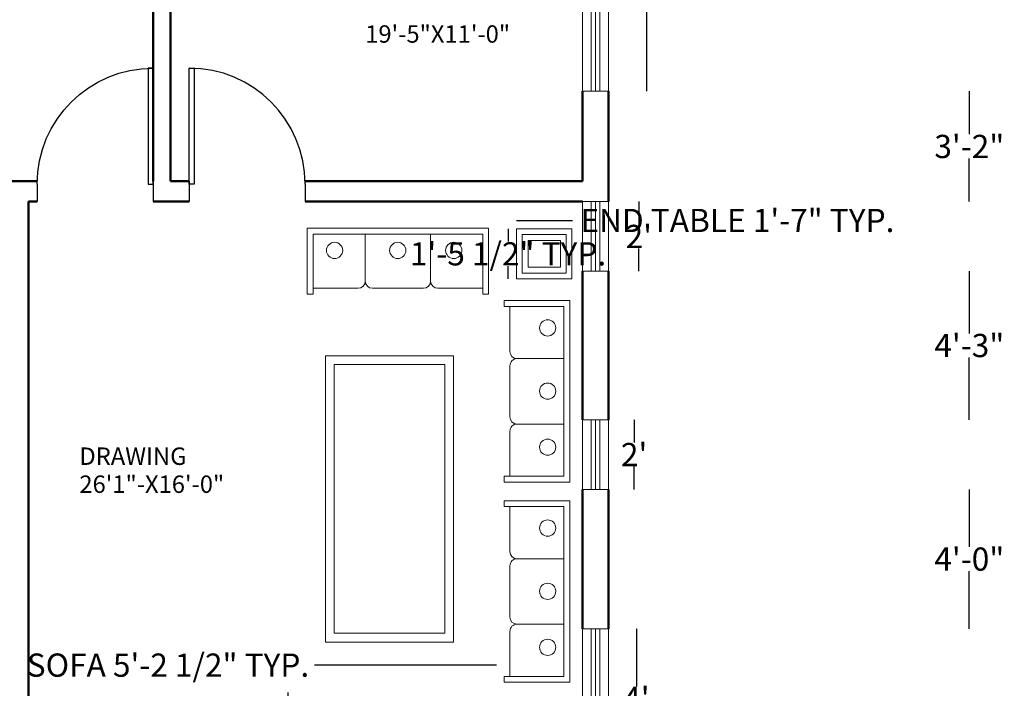
# Model space of a CAD drawing. Units: inches. Extents: x -135167 to -134597, y 156853 to 157819.
# Tile 4 of 5: x -134948 to -134608, y 157306 to 157537. Entities that reach past the tile are written whole.
import ezdxf

# ---------------------------------------------------------------- set-up
doc = ezdxf.new("R2010")
doc.units = ezdxf.units.IN
doc.header["$MEASUREMENT"] = 0
for name, color, linetype, lineweight in [('A-ANNO-DIMS', 4, 'Continuous', 18), ('A-AREA-IDEN', 76, 'Continuous', 25), ('A-FURN', 1, 'Continuous', 18), ('doors', 5, 'Continuous', 25), ('walls', 2, 'Continuous', 50), ('window', 6, 'Continuous', 18)]:
    doc.layers.add(name, color=color, linetype=linetype, lineweight=lineweight)
doc.styles.get("Standard").update_dxf_attribs({"font": 'arial.ttf'})
doc.dimstyles.get("Standard").update_dxf_attribs({"dimtxt": 8, "dimasz": 0.18, "dimexe": 0.18, "dimexo": 0.0625, "dimgap": 0.09, "dimtad": 0, "dimtih": 1, "dimtoh": 1, "dimdec": 0, "dimzin": 0, "dimdsep": 46, "dimlunit": 3, "dimtxsty": 'Standard', "dimblk": 'ARCHTICK', "dimcen": 0.09, "dimse1": 1, "dimse2": 1, "dimadec": 0, "dimazin": 0, "dimtfac": 1, "dimtdec": 0, "dimtofl": 0, "dimtmove": 0, "dimatfit": 3, "dimldrblk": 'DOTSMALL', "dimfxl": 1, "dimtolj": 1, "dimtzin": 0, "dimarcsym": 0})

# ---------------------------------------------------------------- blocks, each defined once
blk = doc.blocks.new('*U6')
for p, q in [((0, 0), (0, -6)), ((40, 0), (40, -6))]:
    blk.add_line(p, q)
blk.add_lwpolyline([(0, 0), (0, 40), (1.75, 40), (1.75, 0)], close=True)
blk.add_arc((0, 0), 40, 0, 90)
blk = doc.blocks.new('_ArchTick')
at = {"color": 0, "linetype": 'ByBlock', "const_width": 0.15}
blk.add_lwpolyline([(-0.5, -0.5), (0.5, 0.5)], dxfattribs=at)
blk = doc.blocks.new('*D25')
at = {"layer": 'A-ANNO-DIMS', "color": 0, "lineweight": -2, "transparency": 16777216}
for p, q in [((-134735.32, 157326.8), (-134735.32, 157306.89)), ((-134735.32, 157278.8), (-134735.32, 157298.71))]:
    blk.add_line(p, q, dxfattribs=at)
at = {"layer": 'Defpoints', "color": 0, "transparency": 16777216}
for p in [(-134747.89, 157326.8), (-134735.32, 157326.8), (-134744.89, 157278.8)]:
    blk.add_point(p, dxfattribs=at)
at = {"layer": 'A-ANNO-DIMS', "color": 0, "lineweight": -2, "transparency": 16777216, "xscale": 0.18, "yscale": 0.18, "zscale": 0.18}
for p, rotation in [((-134735.32, 157326.8), 90), ((-134735.32, 157278.8), 270)]:
    blk.add_blockref('_ArchTick', p, dxfattribs=dict(at, rotation=rotation))
at = {"layer": 'A-ANNO-DIMS', "color": 0, "transparency": 16777216, "insert": (-134735.32, 157302.8), "char_height": 8, "attachment_point": 5}
blk.add_mtext("\\A1;4'", dxfattribs=at)
blk = doc.blocks.new('_DotSmall')
at = {"color": 0, "linetype": 'ByBlock', "const_width": 0.5}
blk.add_lwpolyline([(-0.0625, 0, 1), (0.0625, 0, 1)], format="xyb", close=True, dxfattribs=at)
blk = doc.blocks.new('*D26')
at = {"layer": 'A-ANNO-DIMS', "color": 0, "lineweight": -2, "transparency": 16777216}
for p, q in [((-134736.11, 157398.8), (-134736.11, 157390.91)), ((-134736.11, 157374.8), (-134736.11, 157382.69))]:
    blk.add_line(p, q, dxfattribs=at)
at = {"layer": 'Defpoints', "color": 0, "transparency": 16777216}
for p in [(-134744.89, 157398.8), (-134736.11, 157398.8), (-134744.89, 157374.8)]:
    blk.add_point(p, dxfattribs=at)
at = {"layer": 'A-ANNO-DIMS', "color": 0, "lineweight": -2, "transparency": 16777216, "xscale": 0.18, "yscale": 0.18, "zscale": 0.18}
for p, rotation in [((-134736.11, 157398.8), 90), ((-134736.11, 157374.8), 270)]:
    blk.add_blockref('_ArchTick', p, dxfattribs=dict(at, rotation=rotation))
at = {"layer": 'A-ANNO-DIMS', "color": 0, "transparency": 16777216, "insert": (-134736.11, 157386.8), "char_height": 8, "attachment_point": 5}
blk.add_mtext("\\A1;2'", dxfattribs=at)
blk = doc.blocks.new('*D27')
at = {"layer": 'A-ANNO-DIMS', "color": 0, "lineweight": -2, "transparency": 16777216}
for p, q in [((-134734.49, 157473.94), (-134734.49, 157466.05)), ((-134734.49, 157449.94), (-134734.49, 157457.84))]:
    blk.add_line(p, q, dxfattribs=at)
at = {"layer": 'Defpoints', "color": 0, "transparency": 16777216}
for p in [(-134744.89, 157473.94), (-134734.49, 157473.94), (-134744.89, 157449.94)]:
    blk.add_point(p, dxfattribs=at)
at = {"layer": 'A-ANNO-DIMS', "color": 0, "lineweight": -2, "transparency": 16777216, "xscale": 0.18, "yscale": 0.18, "zscale": 0.18}
for p, rotation in [((-134734.49, 157473.94), 90), ((-134734.49, 157449.94), 270)]:
    blk.add_blockref('_ArchTick', p, dxfattribs=dict(at, rotation=rotation))
at = {"layer": 'A-ANNO-DIMS', "color": 0, "transparency": 16777216, "insert": (-134734.49, 157461.94), "char_height": 8, "attachment_point": 5}
blk.add_mtext("\\A1;2'", dxfattribs=at)
blk = doc.blocks.new('*D28')
at = {"layer": 'A-ANNO-DIMS', "color": 0, "lineweight": -2, "transparency": 16777216}
for p, q in [((-134731.73, 157607.94), (-134731.73, 157564.12)), ((-134731.73, 157511.94), (-134731.73, 157555.77))]:
    blk.add_line(p, q, dxfattribs=at)
at = {"layer": 'Defpoints', "color": 0, "transparency": 16777216}
for p in [(-134744.89, 157607.94), (-134731.73, 157607.94), (-134744.89, 157511.94)]:
    blk.add_point(p, dxfattribs=at)
at = {"layer": 'A-ANNO-DIMS', "color": 0, "lineweight": -2, "transparency": 16777216, "xscale": 0.18, "yscale": 0.18, "zscale": 0.18}
for p, rotation in [((-134731.73, 157607.94), 90), ((-134731.73, 157511.94), 270)]:
    blk.add_blockref('_ArchTick', p, dxfattribs=dict(at, rotation=rotation))
at = {"layer": 'A-ANNO-DIMS', "color": 0, "transparency": 16777216, "insert": (-134731.73, 157559.94), "char_height": 8, "attachment_point": 5}
blk.add_mtext("\\A1;8'", dxfattribs=at)
blk = doc.blocks.new('SOFA-THREE-SEAT')
for p, q in [((20, 4.47), (20, 20.64)), ((42.55, 4.47), (42.55, 20.64)), ((2, 2), (2, 0)), ((60.55, 2), (60.55, 0))]:
    blk.add_line(p, q)
for points in [[(2, 0), (0, 0), (0, 22.64), (62.55, 22.64), (62.55, 0), (60.55, 0)], [(17.53, 2), (2, 2), (2, 20.64), (60.55, 20.64), (60.55, 2), (45.02, 2)], [(40.07, 2), (22.47, 2)]]:
    blk.add_lwpolyline(points)
for centre in [(9.42, 15.02), (31.21, 15.02), (50.51, 15.02)]:
    blk.add_circle(centre, 2.8)
for centre, start, end in [((17.53, 4.47), 270, 0), ((22.47, 4.47), 180, 270), ((40.07, 4.47), 270, 0), ((45.02, 4.47), 180, 270)]:
    blk.add_arc(centre, 2.47, start, end)
blk = doc.blocks.new('TABLE-END')
for points in [[(0, 17.25), (19.14, 17.25), (19.14, 0), (0, 0)], [(2, 15.25), (17.14, 15.25), (17.14, 2), (2, 2)], [(4, 13.25), (15.14, 13.25), (15.14, 4), (4, 4)]]:
    blk.add_lwpolyline(points, close=True)
blk = doc.blocks.new('WIN-96IN')
for p, q in [((0, 96), (9, 96)), ((0, 96), (0, 0)), ((3, 96), (3, 0)), ((4.5, 96), (4.5, 0)), ((6, 96), (6, 0)), ((9, 96), (9, 0)), ((0, 0), (9, 0))]:
    blk.add_line(p, q)
blk = doc.blocks.new('WIN-24IN')
for p, q in [((0, 24), (9, 24)), ((0, 24), (0, 0)), ((3, 24), (3, 0)), ((4.5, 24), (4.5, 0)), ((6, 24), (6, 0)), ((9, 24), (9, 0)), ((0, 0), (9, 0))]:
    blk.add_line(p, q)
blk = doc.blocks.new('WIN-48IN')
for p, q in [((0, 48), (9, 48)), ((0, 0), (0, 48)), ((3, 0), (3, 48)), ((4.5, 0), (4.5, 48)), ((6, 0), (6, 48)), ((9, 0), (9, 48)), ((0, 0), (9, 0))]:
    blk.add_line(p, q)
blk = doc.blocks.new('*D46')
at = {"layer": 'A-ANNO-DIMS', "color": 0, "lineweight": -2, "transparency": 16777216}
for p, q in [((-134846.08, 157314.27), (-134846.26, 157314.27)), ((-134783.53, 157314.27), (-134846.08, 157314.27))]:
    blk.add_line(p, q, dxfattribs=at)
at = {"layer": 'Defpoints', "color": 0, "transparency": 16777216}
for p in [(-134846.08, 157314.27), (-134846.08, 157304.89), (-134783.53, 157304.89)]:
    blk.add_point(p, dxfattribs=at)
at = {"layer": 'A-ANNO-DIMS', "color": 0, "lineweight": -2, "transparency": 16777216, "xscale": 0.18, "yscale": 0.18, "zscale": 0.18, "rotation": 180}
blk.add_blockref('_ArchTick', (-134846.08, 157314.27), dxfattribs=at)
at = {"layer": 'A-ANNO-DIMS', "color": 0, "lineweight": -2, "transparency": 16777216, "xscale": 0.18, "yscale": 0.18, "zscale": 0.18}
blk.add_blockref('_ArchTick', (-134783.53, 157314.27), dxfattribs=at)
at = {"layer": 'A-ANNO-DIMS', "color": 0, "transparency": 16777216, "insert": (-134896.8, 157314.27), "char_height": 8, "attachment_point": 5}
blk.add_mtext('\\A1;SOFA 5\'-2 1/2" TYP.', dxfattribs=at)
blk = doc.blocks.new('*D47')
at = {"layer": 'A-ANNO-DIMS', "color": 0, "lineweight": -2, "transparency": 16777216}
for p, q in [((-134855.46, 157304.89), (-134855.46, 157297.8)), ((-134855.46, 157282.25), (-134855.46, 157289.34))]:
    blk.add_line(p, q, dxfattribs=at)
at = {"layer": 'Defpoints', "color": 0, "transparency": 16777216}
for p in [(-134846.08, 157304.89), (-134855.46, 157282.25), (-134846.08, 157282.25)]:
    blk.add_point(p, dxfattribs=at)
at = {"layer": 'A-ANNO-DIMS', "color": 0, "lineweight": -2, "transparency": 16777216, "xscale": 0.18, "yscale": 0.18, "zscale": 0.18}
for p, rotation in [((-134855.46, 157304.89), 90), ((-134855.46, 157282.25), 270)]:
    blk.add_blockref('_ArchTick', p, dxfattribs=dict(at, rotation=rotation))
at = {"layer": 'A-ANNO-DIMS', "color": 0, "transparency": 16777216, "insert": (-134855.46, 157293.57), "char_height": 8, "attachment_point": 5}
blk.add_mtext('\\A1;1\'-10 1/2" TYP.', dxfattribs=at)
blk = doc.blocks.new('*D50')
at = {"layer": 'A-ANNO-DIMS', "color": 0, "lineweight": -2, "transparency": 16777216}
for p, q in [((-134776.68, 157467.45), (-134757.54, 157467.45)), ((-134757.54, 157467.45), (-134757.36, 157467.45))]:
    blk.add_line(p, q, dxfattribs=at)
at = {"layer": 'Defpoints', "color": 0, "transparency": 16777216}
for p in [(-134757.54, 157467.45), (-134776.68, 157464.58), (-134757.54, 157464.58)]:
    blk.add_point(p, dxfattribs=at)
at = {"layer": 'A-ANNO-DIMS', "color": 0, "lineweight": -2, "transparency": 16777216, "xscale": 0.18, "yscale": 0.18, "zscale": 0.18, "rotation": 180}
blk.add_blockref('_ArchTick', (-134776.68, 157467.45), dxfattribs=at)
at = {"layer": 'A-ANNO-DIMS', "color": 0, "lineweight": -2, "transparency": 16777216, "xscale": 0.18, "yscale": 0.18, "zscale": 0.18}
blk.add_blockref('_ArchTick', (-134757.54, 157467.45), dxfattribs=at)
at = {"layer": 'A-ANNO-DIMS', "color": 0, "transparency": 16777216, "insert": (-134700.49, 157467.45), "char_height": 8, "attachment_point": 5}
blk.add_mtext('\\A1;END TABLE 1\'-7" TYP.', dxfattribs=at)
blk = doc.blocks.new('*D51')
at = {"layer": 'A-ANNO-DIMS', "color": 0, "lineweight": -2, "transparency": 16777216}
for p, q in [((-134779.55, 157464.58), (-134779.55, 157460.18)), ((-134779.55, 157447.33), (-134779.55, 157451.73))]:
    blk.add_line(p, q, dxfattribs=at)
at = {"layer": 'Defpoints', "color": 0, "transparency": 16777216}
for p in [(-134779.55, 157464.58), (-134776.68, 157464.58), (-134776.68, 157447.33)]:
    blk.add_point(p, dxfattribs=at)
at = {"layer": 'A-ANNO-DIMS', "color": 0, "lineweight": -2, "transparency": 16777216, "xscale": 0.18, "yscale": 0.18, "zscale": 0.18}
for p, rotation in [((-134779.55, 157464.58), 90), ((-134779.55, 157447.33), 270)]:
    blk.add_blockref('_ArchTick', p, dxfattribs=dict(at, rotation=rotation))
at = {"layer": 'A-ANNO-DIMS', "color": 0, "transparency": 16777216, "insert": (-134779.55, 157455.95), "char_height": 8, "attachment_point": 5}
blk.add_mtext('\\A1;1\'-5 1/2" TYP.', dxfattribs=at)
blk = doc.blocks.new('*D62')
at = {"layer": 'A-ANNO-DIMS', "color": 0, "lineweight": -2, "transparency": 16777216}
for p, q in [((-134620.54, 157511.94), (-134620.54, 157497.12)), ((-134620.54, 157473.94), (-134620.54, 157488.77))]:
    blk.add_line(p, q, dxfattribs=at)
at = {"layer": 'Defpoints', "color": 0, "transparency": 16777216}
for p in [(-134744.89, 157511.94), (-134744.89, 157473.94), (-134620.54, 157473.94)]:
    blk.add_point(p, dxfattribs=at)
at = {"layer": 'A-ANNO-DIMS', "color": 0, "lineweight": -2, "transparency": 16777216, "xscale": 0.18, "yscale": 0.18, "zscale": 0.18}
for p, rotation in [((-134620.54, 157511.94), 90), ((-134620.54, 157473.94), 270)]:
    blk.add_blockref('_ArchTick', p, dxfattribs=dict(at, rotation=rotation))
at = {"layer": 'A-ANNO-DIMS', "color": 0, "transparency": 16777216, "insert": (-134620.54, 157492.94), "char_height": 8, "attachment_point": 5}
blk.add_mtext('\\A1;3\'-2"', dxfattribs=at)
blk = doc.blocks.new('*D63')
at = {"layer": 'A-ANNO-DIMS', "color": 0, "lineweight": -2, "transparency": 16777216}
for p, q in [((-134620.54, 157449.94), (-134620.54, 157428.55)), ((-134620.54, 157398.8), (-134620.54, 157420.19))]:
    blk.add_line(p, q, dxfattribs=at)
at = {"layer": 'Defpoints', "color": 0, "transparency": 16777216}
for p in [(-134744.89, 157449.94), (-134744.89, 157398.8), (-134620.54, 157398.8)]:
    blk.add_point(p, dxfattribs=at)
at = {"layer": 'A-ANNO-DIMS', "color": 0, "lineweight": -2, "transparency": 16777216, "xscale": 0.18, "yscale": 0.18, "zscale": 0.18}
for p, rotation in [((-134620.54, 157449.94), 90), ((-134620.54, 157398.8), 270)]:
    blk.add_blockref('_ArchTick', p, dxfattribs=dict(at, rotation=rotation))
at = {"layer": 'A-ANNO-DIMS', "color": 0, "transparency": 16777216, "insert": (-134620.54, 157424.37), "char_height": 8, "attachment_point": 5}
blk.add_mtext('\\A1;4\'-3"', dxfattribs=at)
blk = doc.blocks.new('*D64')
at = {"layer": 'A-ANNO-DIMS', "color": 0, "lineweight": -2, "transparency": 16777216}
for p, q in [((-134620.54, 157374.8), (-134620.54, 157354.98)), ((-134620.54, 157326.8), (-134620.54, 157346.63))]:
    blk.add_line(p, q, dxfattribs=at)
at = {"layer": 'Defpoints', "color": 0, "transparency": 16777216}
for p in [(-134744.89, 157374.8), (-134744.89, 157326.8), (-134620.54, 157326.8)]:
    blk.add_point(p, dxfattribs=at)
at = {"layer": 'A-ANNO-DIMS', "color": 0, "lineweight": -2, "transparency": 16777216, "xscale": 0.18, "yscale": 0.18, "zscale": 0.18}
for p, rotation in [((-134620.54, 157374.8), 90), ((-134620.54, 157326.8), 270)]:
    blk.add_blockref('_ArchTick', p, dxfattribs=dict(at, rotation=rotation))
at = {"layer": 'A-ANNO-DIMS', "color": 0, "transparency": 16777216, "insert": (-134620.54, 157350.8), "char_height": 8, "attachment_point": 5}
blk.add_mtext('\\A1;4\'-0"', dxfattribs=at)
blk = doc.blocks.new('*D67')
at = {"layer": 'A-ANNO-DIMS', "color": 0, "lineweight": -2, "transparency": 16777216}
for p, q in [((-134744.89, 157806.8), (-134732.89, 157806.8)), ((-134732.89, 157806.8), (-134732.71, 157806.8))]:
    blk.add_line(p, q, dxfattribs=at)
at = {"layer": 'Defpoints', "color": 0, "transparency": 16777216}
for p in [(-134732.89, 157806.8), (-134744.89, 157145.8), (-134732.89, 157145.8)]:
    blk.add_point(p, dxfattribs=at)
at = {"layer": 'A-ANNO-DIMS', "color": 0, "lineweight": -2, "transparency": 16777216, "xscale": 0.18, "yscale": 0.18, "zscale": 0.18, "rotation": 180}
blk.add_blockref('_ArchTick', (-134744.89, 157806.8), dxfattribs=at)
at = {"layer": 'A-ANNO-DIMS', "color": 0, "lineweight": -2, "transparency": 16777216, "xscale": 0.18, "yscale": 0.18, "zscale": 0.18}
blk.add_blockref('_ArchTick', (-134732.89, 157806.8), dxfattribs=at)
at = {"layer": 'A-ANNO-DIMS', "color": 0, "transparency": 16777216, "insert": (-134722.36, 157806.8), "char_height": 8, "attachment_point": 5}
blk.add_mtext('\\A1;1\'-0"', dxfattribs=at)
blk = doc.blocks.new('*D73')
at = {"layer": 'A-ANNO-DIMS', "color": 0, "lineweight": -2, "transparency": 16777216}
for p, q in [((-134842.49, 157806.8), (-134831.13, 157806.8)), ((-134798.32, 157806.8), (-134809.69, 157806.8))]:
    blk.add_line(p, q, dxfattribs=at)
at = {"layer": 'Defpoints', "color": 0, "transparency": 16777216}
for p in [(-134798.32, 157806.8), (-134842.49, 157420.8), (-134798.32, 157420.8)]:
    blk.add_point(p, dxfattribs=at)
at = {"layer": 'A-ANNO-DIMS', "color": 0, "lineweight": -2, "transparency": 16777216, "xscale": 0.18, "yscale": 0.18, "zscale": 0.18, "rotation": 180}
blk.add_blockref('_ArchTick', (-134842.49, 157806.8), dxfattribs=at)
at = {"layer": 'A-ANNO-DIMS', "color": 0, "lineweight": -2, "transparency": 16777216, "xscale": 0.18, "yscale": 0.18, "zscale": 0.18}
blk.add_blockref('_ArchTick', (-134798.32, 157806.8), dxfattribs=at)
at = {"layer": 'A-ANNO-DIMS', "color": 0, "transparency": 16777216, "insert": (-134820.41, 157806.8), "char_height": 8, "attachment_point": 5}
blk.add_mtext('\\A1;3\'-8"', dxfattribs=at)
blk = doc.blocks.new('*D74')
at = {"layer": 'A-ANNO-DIMS', "color": 0, "lineweight": -2, "transparency": 16777216}
for p, q in [((-135146.24, 157420.8), (-135146.24, 157375.74)), ((-135146.24, 157322.23), (-135146.24, 157367.29))]:
    blk.add_line(p, q, dxfattribs=at)
at = {"layer": 'Defpoints', "color": 0, "transparency": 16777216}
for p in [(-134842.49, 157420.8), (-135146.24, 157322.23), (-134842.49, 157322.23)]:
    blk.add_point(p, dxfattribs=at)
at = {"layer": 'A-ANNO-DIMS', "color": 0, "lineweight": -2, "transparency": 16777216, "xscale": 0.18, "yscale": 0.18, "zscale": 0.18}
for p, rotation in [((-135146.24, 157420.8), 90), ((-135146.24, 157322.23), 270)]:
    blk.add_blockref('_ArchTick', p, dxfattribs=dict(at, rotation=rotation))
at = {"layer": 'A-ANNO-DIMS', "color": 0, "transparency": 16777216, "insert": (-135146.24, 157371.51), "char_height": 8, "attachment_point": 5}
blk.add_mtext('\\A1;8\'-2 1/2"', dxfattribs=at)
blk = doc.blocks.new('*D75')
at = {"layer": 'A-ANNO-DIMS', "color": 0, "lineweight": -2, "transparency": 16777216}
for p, q in [((-135146.24, 157473.94), (-135146.24, 157473.51)), ((-135146.24, 157464.74), (-135146.24, 157465.17))]:
    blk.add_line(p, q, dxfattribs=at)
at = {"layer": 'Defpoints', "color": 0, "transparency": 16777216}
for p in [(-135146.24, 157473.94), (-134849.54, 157473.94), (-134848.8, 157464.74)]:
    blk.add_point(p, dxfattribs=at)
at = {"layer": 'A-ANNO-DIMS', "color": 0, "lineweight": -2, "transparency": 16777216, "xscale": 0.18, "yscale": 0.18, "zscale": 0.18}
for p, rotation in [((-135146.24, 157473.94), 90), ((-135146.24, 157464.74), 270)]:
    blk.add_blockref('_ArchTick', p, dxfattribs=dict(at, rotation=rotation))
at = {"layer": 'A-ANNO-DIMS', "color": 0, "transparency": 16777216, "insert": (-135146.24, 157469.34), "char_height": 8, "attachment_point": 5}
blk.add_mtext('\\A1;0\'-9"', dxfattribs=at)
blk = doc.blocks.new('*D76')
at = {"layer": 'A-ANNO-DIMS', "color": 0, "lineweight": -2, "transparency": 16777216}
for p, q in [((-134786.25, 157806.8), (-134753.89, 157806.8)), ((-134753.89, 157806.8), (-134753.71, 157806.8))]:
    blk.add_line(p, q, dxfattribs=at)
at = {"layer": 'Defpoints', "color": 0, "transparency": 16777216}
for p in [(-134753.89, 157806.8), (-134753.89, 157473.94), (-134786.25, 157464.74)]:
    blk.add_point(p, dxfattribs=at)
at = {"layer": 'A-ANNO-DIMS', "color": 0, "lineweight": -2, "transparency": 16777216, "xscale": 0.18, "yscale": 0.18, "zscale": 0.18, "rotation": 180}
blk.add_blockref('_ArchTick', (-134786.25, 157806.8), dxfattribs=at)
at = {"layer": 'A-ANNO-DIMS', "color": 0, "lineweight": -2, "transparency": 16777216, "xscale": 0.18, "yscale": 0.18, "zscale": 0.18}
blk.add_blockref('_ArchTick', (-134753.89, 157806.8), dxfattribs=at)
at = {"layer": 'A-ANNO-DIMS', "color": 0, "transparency": 16777216, "insert": (-134733.59, 157806.8), "char_height": 8, "attachment_point": 5}
blk.add_mtext('\\A1;2\'-8 1/2"', dxfattribs=at)
blk = doc.blocks.new('*D77')
at = {"layer": 'A-ANNO-DIMS', "color": 0, "lineweight": -2, "transparency": 16777216}
for p, q in [((-134798.32, 157806.8), (-134780.93, 157806.8)), ((-134780.93, 157806.8), (-134780.75, 157806.8))]:
    blk.add_line(p, q, dxfattribs=at)
at = {"layer": 'Defpoints', "color": 0, "transparency": 16777216}
for p in [(-134780.93, 157806.8), (-134798.32, 157322.23), (-134780.93, 157308.36)]:
    blk.add_point(p, dxfattribs=at)
at = {"layer": 'A-ANNO-DIMS', "color": 0, "lineweight": -2, "transparency": 16777216, "xscale": 0.18, "yscale": 0.18, "zscale": 0.18, "rotation": 180}
blk.add_blockref('_ArchTick', (-134798.32, 157806.8), dxfattribs=at)
at = {"layer": 'A-ANNO-DIMS', "color": 0, "lineweight": -2, "transparency": 16777216, "xscale": 0.18, "yscale": 0.18, "zscale": 0.18}
blk.add_blockref('_ArchTick', (-134780.93, 157806.8), dxfattribs=at)
at = {"layer": 'A-ANNO-DIMS', "color": 0, "transparency": 16777216, "insert": (-134761.09, 157806.8), "char_height": 8, "attachment_point": 5}
blk.add_mtext('\\A1;1\'-5 1/2"', dxfattribs=at)
blk = doc.blocks.new('*D78')
at = {"layer": 'A-ANNO-DIMS', "color": 0, "lineweight": -2, "transparency": 16777216}
for p, q in [((-135146.24, 157442.1), (-135146.24, 157435.68)), ((-135146.24, 157420.8), (-135146.24, 157427.22))]:
    blk.add_line(p, q, dxfattribs=at)
at = {"layer": 'Defpoints', "color": 0, "transparency": 16777216}
for p in [(-135146.24, 157442.1), (-134848.8, 157442.1), (-134842.49, 157420.8)]:
    blk.add_point(p, dxfattribs=at)
at = {"layer": 'A-ANNO-DIMS', "color": 0, "lineweight": -2, "transparency": 16777216, "xscale": 0.18, "yscale": 0.18, "zscale": 0.18}
for p, rotation in [((-135146.24, 157442.1), 90), ((-135146.24, 157420.8), 270)]:
    blk.add_blockref('_ArchTick', p, dxfattribs=dict(at, rotation=rotation))
at = {"layer": 'A-ANNO-DIMS', "color": 0, "transparency": 16777216, "insert": (-135146.24, 157431.45), "char_height": 8, "attachment_point": 5}
blk.add_mtext('\\A1;1\'-9 1/2"', dxfattribs=at)
blk = doc.blocks.new('*D81')
at = {"layer": 'A-ANNO-DIMS', "color": 0, "lineweight": -2, "transparency": 16777216}
for p, q in [((-134941.89, 156858.2), (-134932.61, 156858.2)), ((-134901.89, 156858.2), (-134911.17, 156858.2))]:
    blk.add_line(p, q, dxfattribs=at)
at = {"layer": 'Defpoints', "color": 0, "transparency": 16777216}
for p in [(-134941.89, 157473.94), (-134901.89, 157473.94), (-134901.89, 156858.2)]:
    blk.add_point(p, dxfattribs=at)
at = {"layer": 'A-ANNO-DIMS', "color": 0, "lineweight": -2, "transparency": 16777216, "xscale": 0.18, "yscale": 0.18, "zscale": 0.18, "rotation": 180}
blk.add_blockref('_ArchTick', (-134941.89, 156858.2), dxfattribs=at)
at = {"layer": 'A-ANNO-DIMS', "color": 0, "lineweight": -2, "transparency": 16777216, "xscale": 0.18, "yscale": 0.18, "zscale": 0.18}
blk.add_blockref('_ArchTick', (-134901.89, 156858.2), dxfattribs=at)
at = {"layer": 'A-ANNO-DIMS', "color": 0, "transparency": 16777216, "insert": (-134921.89, 156858.2), "char_height": 8, "attachment_point": 5}
blk.add_mtext('\\A1;3\'-4"', dxfattribs=at)
blk = doc.blocks.new('*D82')
at = {"layer": 'A-ANNO-DIMS', "color": 0, "lineweight": -2, "transparency": 16777216}
for p, q in [((-134889.54, 156858.2), (-134880.26, 156858.2)), ((-134849.54, 156858.2), (-134858.82, 156858.2))]:
    blk.add_line(p, q, dxfattribs=at)
at = {"layer": 'Defpoints', "color": 0, "transparency": 16777216}
for p in [(-134889.54, 157473.94), (-134849.54, 157473.94), (-134849.54, 156858.2)]:
    blk.add_point(p, dxfattribs=at)
at = {"layer": 'A-ANNO-DIMS', "color": 0, "lineweight": -2, "transparency": 16777216, "xscale": 0.18, "yscale": 0.18, "zscale": 0.18, "rotation": 180}
blk.add_blockref('_ArchTick', (-134889.54, 156858.2), dxfattribs=at)
at = {"layer": 'A-ANNO-DIMS', "color": 0, "lineweight": -2, "transparency": 16777216, "xscale": 0.18, "yscale": 0.18, "zscale": 0.18}
blk.add_blockref('_ArchTick', (-134849.54, 156858.2), dxfattribs=at)
at = {"layer": 'A-ANNO-DIMS', "color": 0, "transparency": 16777216, "insert": (-134869.54, 156858.2), "char_height": 8, "attachment_point": 5}
blk.add_mtext('\\A1;3\'-4"', dxfattribs=at)
blk = doc.blocks.new('*D90')
at = {"layer": 'A-ANNO-DIMS', "color": 0, "lineweight": -2, "transparency": 16777216}
for p, q in [((-134791.39, 157806.8), (-134756.89, 157806.8)), ((-134756.89, 157806.8), (-134756.71, 157806.8))]:
    blk.add_line(p, q, dxfattribs=at)
at = {"layer": 'Defpoints', "color": 0, "transparency": 16777216}
for p in [(-134756.89, 157806.8), (-134791.39, 156969.8), (-134756.89, 156969.8)]:
    blk.add_point(p, dxfattribs=at)
at = {"layer": 'A-ANNO-DIMS', "color": 0, "lineweight": -2, "transparency": 16777216, "xscale": 0.18, "yscale": 0.18, "zscale": 0.18, "rotation": 180}
blk.add_blockref('_ArchTick', (-134791.39, 157806.8), dxfattribs=at)
at = {"layer": 'A-ANNO-DIMS', "color": 0, "lineweight": -2, "transparency": 16777216, "xscale": 0.18, "yscale": 0.18, "zscale": 0.18}
blk.add_blockref('_ArchTick', (-134756.89, 157806.8), dxfattribs=at)
at = {"layer": 'A-ANNO-DIMS', "color": 0, "transparency": 16777216, "insert": (-134733.49, 157806.8), "char_height": 8, "attachment_point": 5}
blk.add_mtext('\\A1;2\'-10 1/2"', dxfattribs=at)
blk = doc.blocks.new('*D92')
at = {"layer": 'A-ANNO-DIMS', "color": 0, "lineweight": -2, "transparency": 16777216}
for p, q in [((-134987.89, 156858.2), (-134955.58, 156858.2)), ((-134901.89, 156858.2), (-134934.2, 156858.2))]:
    blk.add_line(p, q, dxfattribs=at)
at = {"layer": 'Defpoints', "color": 0, "transparency": 16777216}
for p in [(-134987.89, 157647.94), (-134901.89, 157647.94), (-134901.89, 156858.2)]:
    blk.add_point(p, dxfattribs=at)
at = {"layer": 'A-ANNO-DIMS', "color": 0, "lineweight": -2, "transparency": 16777216, "xscale": 0.18, "yscale": 0.18, "zscale": 0.18, "rotation": 180}
blk.add_blockref('_ArchTick', (-134987.89, 156858.2), dxfattribs=at)
at = {"layer": 'A-ANNO-DIMS', "color": 0, "lineweight": -2, "transparency": 16777216, "xscale": 0.18, "yscale": 0.18, "zscale": 0.18}
blk.add_blockref('_ArchTick', (-134901.89, 156858.2), dxfattribs=at)
at = {"layer": 'A-ANNO-DIMS', "color": 0, "transparency": 16777216, "insert": (-134944.89, 156858.2), "char_height": 8, "attachment_point": 5}
blk.add_mtext('\\A1;7\'-2"', dxfattribs=at)

msp = doc.modelspace()

# ---------------------------------------------------------------- linework, layer by layer
at = {"layer": 'A-FURN'}
for points in [[(-134842.49, 157420.8), (-134798.32, 157420.8), (-134798.32, 157322.23), (-134842.49, 157322.23)], [(-134839.49, 157417.8), (-134801.32, 157417.8), (-134801.32, 157325.23), (-134839.49, 157325.23)]]:
    msp.add_lwpolyline(points, close=True, dxfattribs=at)
at = {"layer": 'doors'}
for p, q in [((-134901.89, 157480.94), (-134901.89, 157473.94)), ((-134889.54, 157480.94), (-134889.54, 157473.94))]:
    msp.add_line(p, q, dxfattribs=at)
at = {"layer": 'walls'}
for p, q in [((-134901.89, 157480.94), (-134901.89, 157641.94)), ((-134895.89, 157480.94), (-134895.89, 157638.94)), ((-134753.89, 157480.94), (-134753.89, 157511.94)), ((-134744.89, 157473.94), (-134744.89, 157511.94)), ((-134962.89, 157480.94), (-134941.87, 157480.94)), ((-134895.89, 157480.94), (-134889.54, 157480.94)), ((-134849.55, 157480.94), (-134753.89, 157480.94)), ((-134944.89, 157176.94), (-134944.89, 157473.94)), ((-134944.89, 157473.94), (-134941.89, 157473.94)), ((-134901.89, 157473.94), (-134889.54, 157473.94)), ((-134849.54, 157473.94), (-134753.89, 157473.94)), ((-134753.89, 157398.8), (-134753.89, 157449.94)), ((-134744.89, 157398.8), (-134744.89, 157449.94)), ((-134753.89, 157326.8), (-134753.89, 157374.8)), ((-134744.89, 157326.8), (-134744.89, 157374.8))]:
    msp.add_line(p, q, dxfattribs=at)

# ---------------------------------------------------------------- block references
at = {"layer": 'A-FURN'}
for name, p in [('SOFA-THREE-SEAT', (-134848.8, 157442.1)), ('TABLE-END', (-134776.68, 157447.33))]:
    msp.add_blockref(name, p, dxfattribs=at)
for p, rotation in [((-134780.93, 157439.86), 269.9999999999994), ((-134780.93, 157370.91), 269.9999999999783)]:
    msp.add_blockref('SOFA-THREE-SEAT', p, dxfattribs=dict(at, rotation=rotation))
at = {"layer": 'doors', "xscale": -1}
msp.add_blockref('*U6', (-134901.89, 157479.94), dxfattribs=at)
at = {"layer": 'doors'}
msp.add_blockref('*U6', (-134889.54, 157479.94), dxfattribs=at)
at = {"layer": 'window'}
for name, p in [('WIN-96IN', (-134753.89, 157511.94)), ('WIN-24IN', (-134753.89, 157449.94))]:
    msp.add_blockref(name, p, dxfattribs=at)
at = {"layer": 'window', "rotation": 180}
for name, p in [('WIN-24IN', (-134744.89, 157398.8)), ('WIN-48IN', (-134744.89, 157326.8))]:
    msp.add_blockref(name, p, dxfattribs=at)

# ---------------------------------------------------------------- texts
at = {"layer": 'A-AREA-IDEN'}
for s, p in [('19\'-5"X11\'-0"', (-134828.8, 157528.68)), ('DRAWING ', (-134927.35, 157383.24)), ('26\'1"-X16\'-0"', (-134927.35, 157373.6))]:
    msp.add_text(s, height=6, dxfattribs=at).set_placement(p)

# ---------------------------------------------------------------- dimensions: what is measured, and where the dimension line sits
at = {"layer": 'A-ANNO-DIMS'}
for base, p1, p2, picture, middle in [((-134780.93, 157806.8), (-134798.32, 157322.23), (-134780.93, 157308.36), '*D77', (-134761.09, 157806.8)), ((-134756.89, 157806.8), (-134791.39, 156969.8), (-134756.89, 156969.8), '*D90', (-134733.49, 157806.8)), ((-134753.89, 157806.8), (-134786.25, 157464.74), (-134753.89, 157473.94), '*D76', (-134733.59, 157806.8)), ((-134798.32, 157806.8), (-134842.49, 157420.8), (-134798.32, 157420.8), '*D73', (-134820.41, 157806.8)), ((-134732.89, 157806.8), (-134744.89, 157145.8), (-134732.89, 157145.8), '*D67', (-134722.36, 157806.8)), ((-134901.89, 156858.2), (-134987.89, 157647.94), (-134901.89, 157647.94), '*D92', (-134944.89, 156858.2)), ((-134901.89, 156858.2), (-134941.89, 157473.94), (-134901.89, 157473.94), '*D81', (-134921.89, 156858.2)), ((-134849.54, 156858.2), (-134889.54, 157473.94), (-134849.54, 157473.94), '*D82', (-134869.54, 156858.2))]:
    dim = msp.add_linear_dim(base=base, p1=p1, p2=p2, dimstyle='Standard', override={"dimdec": 1, "dimlfac": 1, "dimrnd": 0, "dimzin": 1, "dimdsep": 46, "dimlunit": 4, "dimfrac": 2}, dxfattribs=at)
    dim.commit()
    dim.dimension.update_dxf_attribs({"geometry": picture, "text_midpoint": middle})
for base, p1, p2, override, picture, middle in [((-134731.73, 157607.94), (-134744.89, 157511.94), (-134744.89, 157607.94), {"dimclrd": 0, "dimclre": 0, "dimclrt": 0}, '*D28', (-134731.73, 157559.94)), ((-134620.54, 157473.94), (-134744.89, 157511.94), (-134744.89, 157473.94), {"dimdec": 1, "dimlfac": 1, "dimrnd": 0, "dimzin": 1, "dimdsep": 46, "dimlunit": 4, "dimfrac": 2}, '*D62', (-134620.54, 157492.94)), ((-135146.24, 157473.94), (-134848.8, 157464.74), (-134849.54, 157473.94), {"dimdec": 1, "dimlfac": 1, "dimrnd": 0, "dimzin": 1, "dimdsep": 46, "dimlunit": 4, "dimfrac": 2}, '*D75', (-135146.24, 157469.34)), ((-134734.49, 157473.94), (-134744.89, 157449.94), (-134744.89, 157473.94), {"dimclrd": 0, "dimclre": 0, "dimclrt": 0}, '*D27', (-134734.49, 157461.94)), ((-134620.54, 157398.8), (-134744.89, 157449.94), (-134744.89, 157398.8), {"dimdec": 1, "dimlfac": 1, "dimrnd": 0, "dimzin": 1, "dimdsep": 46, "dimlunit": 4, "dimfrac": 2}, '*D63', (-134620.54, 157424.37)), ((-135146.24, 157442.1), (-134842.49, 157420.8), (-134848.8, 157442.1), {"dimdec": 1, "dimlfac": 1, "dimrnd": 0, "dimzin": 1, "dimdsep": 46, "dimlunit": 4, "dimfrac": 2}, '*D78', (-135146.24, 157431.45)), ((-135146.24, 157322.23), (-134842.49, 157420.8), (-134842.49, 157322.23), {"dimdec": 1, "dimlfac": 1, "dimrnd": 0, "dimzin": 1, "dimdsep": 46, "dimlunit": 4, "dimfrac": 2}, '*D74', (-135146.24, 157371.51)), ((-134736.11, 157398.8), (-134744.89, 157374.8), (-134744.89, 157398.8), {"dimclrd": 0, "dimclre": 0, "dimclrt": 0}, '*D26', (-134736.11, 157386.8)), ((-134620.54, 157326.8), (-134744.89, 157374.8), (-134744.89, 157326.8), {"dimdec": 1, "dimlfac": 1, "dimrnd": 0, "dimzin": 1, "dimdsep": 46, "dimlunit": 4, "dimfrac": 2}, '*D64', (-134620.54, 157350.8)), ((-134735.32, 157326.8), (-134744.89, 157278.8), (-134747.89, 157326.8), {"dimclrd": 0, "dimclre": 0, "dimclrt": 0}, '*D25', (-134735.32, 157302.8))]:
    dim = msp.add_linear_dim(base=base, p1=p1, p2=p2, angle=90, dimstyle='Standard', override=override, dxfattribs=at)
    dim.commit()
    dim.dimension.update_dxf_attribs({"geometry": picture, "text_midpoint": middle})
dim = msp.add_linear_dim(base=(-134757.54, 157467.45), p1=(-134776.68, 157464.58), p2=(-134757.54, 157464.58), text='END TABLE <> TYP.', dimstyle='Standard', override={"dimdec": 1, "dimlfac": 1, "dimrnd": 0, "dimzin": 1, "dimdsep": 46, "dimlunit": 4, "dimfrac": 2}, dxfattribs=at)
dim.commit()
dim.dimension.update_dxf_attribs({"geometry": '*D50', "text_midpoint": (-134700.49, 157467.45)})
for base, p1, p2, angle, text, picture, middle in [((-134779.5513, 157464.5786), (-134776.6805, 157447.3264), (-134776.6805, 157464.5786), 90, '<> TYP.', '*D51', (-134779.5513, 157455.9525)), ((-134846.0812, 157314.271), (-134783.5338, 157304.8889), (-134846.0812, 157304.8889), 180, 'SOFA <> TYP.', '*D46', (-134896.8014, 157314.271)), ((-134855.46, 157282.25), (-134846.08, 157304.89), (-134846.08, 157282.25), 270, '<> TYP.', '*D47', (-134855.46, 157293.57))]:
    dim = msp.add_linear_dim(base=base, p1=p1, p2=p2, angle=angle, text=text, dimstyle='Standard', override={"dimdec": 1, "dimlfac": 1, "dimrnd": 0, "dimzin": 1, "dimdsep": 46, "dimlunit": 4, "dimfrac": 2}, dxfattribs=at)
    dim.commit()
    dim.dimension.update_dxf_attribs({"geometry": picture, "text_midpoint": middle})

doc.saveas('drawing.dxf')
